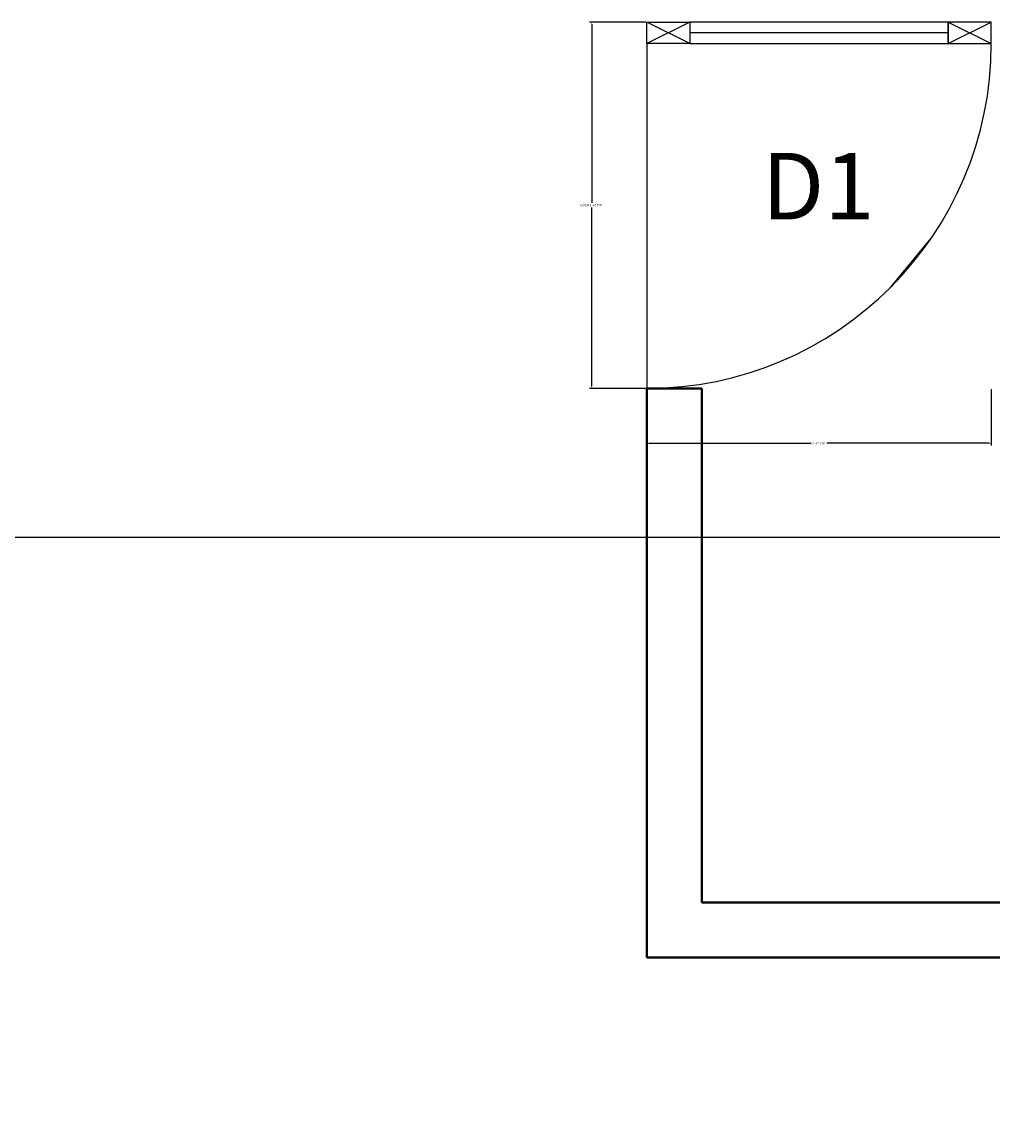
# Model space of a CAD drawing. Units: inches. Extents: x 182 to 1022, y -617 to 111.
# Tile 29 of 33: x 836 to 915, y -337 to -246. Entities that reach past the tile are written whole.
import ezdxf

# ---------------------------------------------------------------- set-up
doc = ezdxf.new("R2010")
doc.units = ezdxf.units.IN
doc.header["$MEASUREMENT"] = 0
for name, color, linetype, lineweight in [('A-ANNO-DIMS', 2, 'Continuous', 18), ('A-ANNO-IDEN', 1, 'Continuous', 18), ('door', 2, 'Continuous', 25), ('wall', 1, 'Continuous', 40)]:
    doc.layers.add(name, color=color, linetype=linetype, lineweight=lineweight)
doc.styles.get("Standard").update_dxf_attribs({"font": 'arial.ttf'})
doc.dimstyles.get("Standard").update_dxf_attribs({"dimtxt": 0.18, "dimasz": 0.18, "dimexe": 0.18, "dimexo": 0.0625, "dimgap": 0.09, "dimtad": 0, "dimtih": 1, "dimtoh": 1, "dimdec": 1, "dimzin": 0, "dimdsep": 46, "dimlunit": 4, "dimtxsty": 'Standard', "dimcen": 0.09, "dimadec": 0, "dimazin": 0, "dimtfac": 1, "dimtdec": 1, "dimtofl": 0, "dimtmove": 0, "dimatfit": 3, "dimfxl": 1, "dimtolj": 1, "dimtzin": 0, "dimarcsym": 0})

# ---------------------------------------------------------------- blocks, each defined once
blk = doc.blocks.new('A$C2D7661C6')
for p, q in [((0, 700), (50, 800)), ((50, 700), (0, 800)), ((25, 700), (25, 100)), ((50, 100), (0, 0)), ((0, 100), (50, 0))]:
    blk.add_line(p, q)
for points in [[(0, 700), (50, 700), (50, 800), (0, 800)], [(0, 100), (50, 100), (50, 700), (0, 700)], [(0, 100), (50, 100), (50, 0), (0, 0)]]:
    blk.add_lwpolyline(points, close=True)
blk.add_arc((50, 0), 800, 0, 90)
blk = doc.blocks.new('A$C7F556C88')
for p, q in [((615.7, 565.7), (500.3, 661.3)), ((50, 0), (850, 0))]:
    blk.add_line(p, q)
blk.add_blockref('A$C2D7661C6', (0, 0))
blk = doc.blocks.new('*D16')
at = {"layer": 'A-ANNO-DIMS', "color": 0, "lineweight": -2, "transparency": 16777216}
for p, q in [((886.742, -246.44), (882.135, -246.44)), ((882.315, -246.62), (882.315, -261.223)), ((882.315, -276.193), (882.315, -261.59)), ((886.742, -276.373), (882.135, -276.373))]:
    blk.add_line(p, q, dxfattribs=at)
at = {"layer": 'A-ANNO-DIMS', "color": 0, "transparency": 16777216}
for points in [[(882.285, -246.62), (882.345, -246.62), (882.315, -246.44)], [(882.285, -276.193), (882.345, -276.193), (882.315, -276.373)]]:
    blk.add_solid(points, dxfattribs=at)
at = {"layer": 'Defpoints', "color": 0, "transparency": 16777216}
for p in [(886.805, -246.44), (882.315, -276.373), (886.805, -276.373)]:
    blk.add_point(p, dxfattribs=at)
at = {"layer": 'A-ANNO-DIMS', "color": 0, "transparency": 16777216, "insert": (882.315, -261.406), "char_height": 0.18, "attachment_point": 5}
blk.add_mtext('\\A1;DOOR 2\'-6" TYP.', dxfattribs=at)
blk = doc.blocks.new('*D17')
at = {"layer": 'A-ANNO-DIMS', "color": 0, "lineweight": -2, "transparency": 16777216}
for p, q in [((886.805, -276.436), (886.805, -281.043)), ((914.977, -276.436), (914.977, -281.043)), ((886.985, -280.863), (900.251, -280.863)), ((914.797, -280.863), (901.531, -280.863))]:
    blk.add_line(p, q, dxfattribs=at)
at = {"layer": 'A-ANNO-DIMS', "color": 0, "transparency": 16777216}
for points in [[(886.985, -280.833), (886.985, -280.893), (886.805, -280.863)], [(914.797, -280.833), (914.797, -280.893), (914.977, -280.863)]]:
    blk.add_solid(points, dxfattribs=at)
at = {"layer": 'Defpoints', "color": 0, "transparency": 16777216}
for p in [(886.805, -276.373), (914.977, -276.373), (914.977, -280.863)]:
    blk.add_point(p, dxfattribs=at)
at = {"layer": 'A-ANNO-DIMS', "color": 0, "transparency": 16777216, "insert": (900.891, -280.863), "char_height": 0.18, "attachment_point": 5}
blk.add_mtext('\\A1;2\'-4" TYP.', dxfattribs=at)
blk = doc.blocks.new('*D39')
at = {"layer": 'A-ANNO-DIMS', "color": 0, "lineweight": -2, "transparency": 16777216}
for p, q in [((238.398, -288.54), (1015.285, -288.54)), ((1015.105, -288.72), (1015.105, -346.775)), ((1015.105, -405.193), (1015.105, -347.138)), ((238.427, -405.373), (1015.285, -405.373))]:
    blk.add_line(p, q, dxfattribs=at)
at = {"layer": 'A-ANNO-DIMS', "color": 0, "transparency": 16777216}
for points in [[(1015.075, -288.72), (1015.135, -288.72), (1015.105, -288.54)], [(1015.075, -405.193), (1015.135, -405.193), (1015.105, -405.373)]]:
    blk.add_solid(points, dxfattribs=at)
at = {"layer": 'Defpoints', "color": 0, "transparency": 16777216}
for p in [(238.335, -288.54), (1015.105, -288.54), (238.364, -405.373)]:
    blk.add_point(p, dxfattribs=at)
at = {"layer": 'A-ANNO-DIMS', "color": 0, "transparency": 16777216, "insert": (1015.105, -346.956), "char_height": 0.18, "attachment_point": 5}
blk.add_mtext('\\A1;9\'-9"', dxfattribs=at)

msp = doc.modelspace()

# ---------------------------------------------------------------- linework, layer by layer
at = {"layer": 'wall'}
for p, q in [((886.805, -276.373), (886.805, -322.873)), ((886.805, -276.373), (891.305, -276.373)), ((891.305, -276.373), (891.305, -318.373)), ((891.305, -318.373), (963.305, -318.373)), ((886.805, -322.873), (963.305, -322.873))]:
    msp.add_line(p, q, dxfattribs=at)

# ---------------------------------------------------------------- block references
at = {"layer": 'door', "xscale": 0.0352158668681478, "yscale": 0.0352158668681478, "zscale": 0.0352158668681478, "rotation": 270}
msp.add_blockref('A$C7F556C88', (886.805, -246.44), dxfattribs=at)

# ---------------------------------------------------------------- texts
at = {"layer": 'A-ANNO-IDEN'}
msp.add_text('D1', height=5.4442, dxfattribs=at).set_placement((896.212, -262.572))

# ---------------------------------------------------------------- dimensions: what is measured, and where the dimension line sits
at = {"layer": 'A-ANNO-DIMS'}
dim = msp.add_linear_dim(base=(882.315, -276.373), p1=(886.805, -246.44), p2=(886.805, -276.373), angle=270, text='DOOR <> TYP.', dimstyle='Standard', override={"dimdec": 1, "dimlfac": 1, "dimrnd": 0, "dimzin": 1, "dimdsep": 46, "dimlunit": 4, "dimfrac": 2}, dxfattribs=at)
dim.commit()
dim.dimension.update_dxf_attribs({"geometry": '*D16', "text_midpoint": (882.315, -261.406)})
dim = msp.add_linear_dim(base=(914.977, -280.863), p1=(886.805, -276.373), p2=(914.977, -276.373), text='<> TYP.', dimstyle='Standard', override={"dimdec": 1, "dimlfac": 1, "dimrnd": 0, "dimzin": 1, "dimdsep": 46, "dimlunit": 4, "dimfrac": 2}, dxfattribs=at)
dim.commit()
dim.dimension.update_dxf_attribs({"geometry": '*D17', "text_midpoint": (900.891, -280.863)})
dim = msp.add_linear_dim(base=(1015.105, -288.54), p1=(238.364, -405.373), p2=(238.335, -288.54), angle=90, dimstyle='Standard', override={"dimdec": 1, "dimlfac": 1, "dimrnd": 0, "dimzin": 1, "dimdsep": 46, "dimlunit": 4, "dimfrac": 2}, dxfattribs=at)
dim.commit()
dim.dimension.update_dxf_attribs({"geometry": '*D39', "text_midpoint": (1015.105, -346.956)})

doc.saveas('drawing.dxf')
